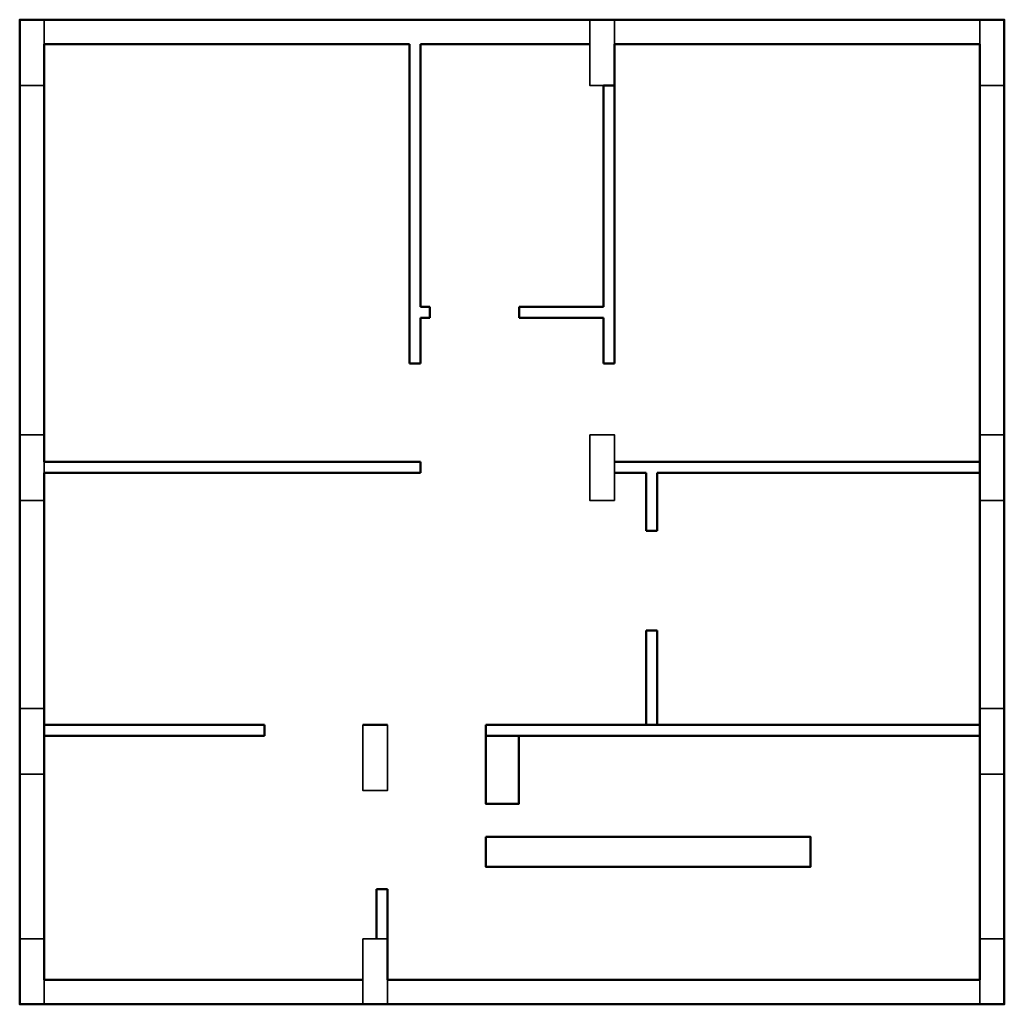
# Model space of a CAD drawing. Units: inches. Extents: x 2160 to 4339, y 1832 to 4384.
# Tile 1 of 1: x 2160.4 to 2520.4, y 1832 to 2192. Entities that reach past the tile are written whole.
import ezdxf

# ---------------------------------------------------------------- set-up
doc = ezdxf.new("R2010")
doc.units = ezdxf.units.IN
doc.layers.add('A-COLS', color=6, linetype='Continuous', lineweight=35)
doc.layers.add('A-WALL', color=7, linetype='Continuous', lineweight=50)

# ---------------------------------------------------------------- blocks, each defined once
blk = doc.blocks.new('COLUMN-230X600')
blk.add_lwpolyline([(2160.37, 2192.01), (2169.37, 2192.01), (2169.37, 2168.01), (2160.37, 2168.01)], close=True)

msp = doc.modelspace()

# ---------------------------------------------------------------- linework, layer by layer
at = {"layer": 'A-WALL'}
for p, q in [((2306.94, 2183.01), (2306.94, 2087.01)), ((2306.94, 2183.01), (2306.94, 2087.01)), ((2373.8, 2168.01), (2373.8, 2087.01)), ((2373.8, 2168.01), (2377.8, 2168.01)), ((2306.94, 2087.01), (2310.28, 2087.01)), ((2306.94, 2087.01), (2310.28, 2087.01)), ((2310.28, 2087.01), (2310.28, 2083.01)), ((2342.94, 2087.01), (2342.94, 2083.01)), ((2342.94, 2083.01), (2342.94, 2087.01)), ((2342.94, 2087.01), (2373.8, 2087.01)), ((2306.94, 2083.01), (2310.28, 2083.01)), ((2306.94, 2083.01), (2306.94, 2066.31)), ((2342.94, 2083.01), (2373.8, 2083.01)), ((2373.8, 2083.01), (2373.8, 2066.31)), ((2373.8, 2066.31), (2373.8, 2083.01)), ((2302.94, 2066.31), (2306.94, 2066.31)), ((2373.8, 2066.31), (2377.8, 2066.31)), ((2377.8, 2066.31), (2373.8, 2066.31)), ((2306.94, 2030.31), (2306.94, 2026.31)), ((2511.37, 2026.31), (2511.37, 2030.31)), ((2377.8, 2026.31), (2389.46, 2026.31)), ((2393.46, 2026.31), (2511.37, 2026.31)), ((2393.46, 2026.31), (2393.46, 2005.09)), ((2393.46, 1968.72), (2393.46, 1934.17)), ((2249.84, 1934.17), (2249.84, 1930.17)), ((2330.84, 1934.17), (2330.84, 1930.17)), ((2389.46, 1934.17), (2511.37, 1934.17)), ((2393.46, 1930.17), (2511.37, 1930.17)), ((2290.84, 1856.01), (2290.84, 1874.17)), ((2290.84, 1874.17), (2294.84, 1874.17)), ((2294.84, 1841.01), (2294.84, 1874.17))]:
    msp.add_line(p, q, dxfattribs=at)
for points in [[(2160.37, 2192.01), (2520.37, 2192.01), (2520.37, 1832.01), (2160.37, 1832.01)], [(2160.37, 1832.01), (2520.37, 1832.01), (2520.37, 2192.01), (2160.37, 2192.01)], [(2330.84, 1930.17), (2342.82, 1930.17), (2342.82, 1905.25), (2330.84, 1905.25)], [(2330.84, 1893.25), (2449.5, 1893.25), (2449.5, 1882.25), (2330.84, 1882.25)]]:
    msp.add_lwpolyline(points, close=True, dxfattribs=at)
for points in [[(2169.37, 2030.31), (2169.37, 2183.01), (2302.94, 2183.01)], [(2377.8, 2183.01), (2511.37, 2183.01), (2511.37, 1841.01), (2294.84, 1841.01)], [(2302.94, 2183.01), (2302.94, 2066.31)], [(2306.94, 2183.01), (2368.8, 2183.01)], [(2377.8, 2183.01), (2377.8, 2066.31)], [(2169.37, 2030.31), (2306.94, 2030.31)], [(2377.8, 2030.31), (2511.37, 2030.31)], [(2285.84, 1841.01), (2169.37, 1841.01), (2169.37, 2026.31)], [(2249.84, 1934.17), (2169.37, 1934.17), (2169.37, 2026.31), (2306.94, 2026.31)], [(2389.46, 2026.31), (2389.46, 2005.09)], [(2389.46, 2005.09), (2393.46, 2005.09)], [(2389.46, 1968.72), (2389.46, 1934.17), (2330.84, 1934.17)], [(2393.46, 1968.72), (2389.46, 1968.72)], [(2294.84, 1934.17), (2285.84, 1934.17)], [(2249.84, 1930.17), (2169.37, 1930.17)], [(2393.46, 1930.17), (2330.84, 1930.17)]]:
    msp.add_lwpolyline(points, dxfattribs=at)

# ---------------------------------------------------------------- block references
at = {"layer": 'A-COLS'}
for p in [(0, 0), (208.43, 0), (0, -151.78), (208.43, -151.74), (0, -251.81), (125.47, -257.84), (0, -336), (125.47, -336)]:
    msp.add_blockref('COLUMN-230X600', p, dxfattribs=at)
at = {"layer": 'A-COLS', "extrusion": (0, 0, -1), "zscale": -1}
for p in [(-4680.74, 0), (-4680.74, -151.78), (-4680.74, -251.81), (-4680.74, -336)]:
    msp.add_blockref('COLUMN-230X600', p, dxfattribs=at)

doc.saveas('drawing.dxf')
